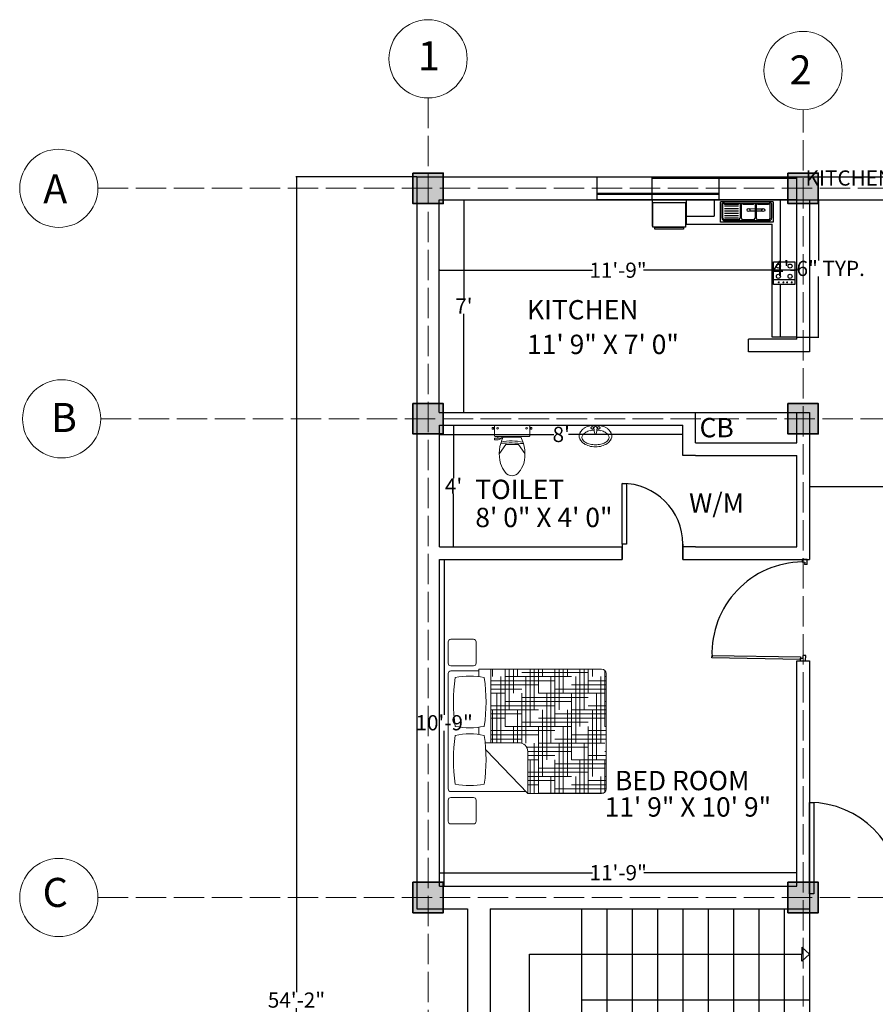
# Model space of a CAD drawing. Units: inches. Extents: x -113 to 5399, y -1393 to 3302.
# Tile 36 of 40: x 3074 to 3412, y 2903 to 3292. Entities that reach past the tile are written whole.
import ezdxf

# ---------------------------------------------------------------- set-up
doc = ezdxf.new("R2010")
doc.units = ezdxf.units.IN
doc.header["$MEASUREMENT"] = 0
doc.linetypes.add('ACAD_ISO02W100', pattern=[15, 12, -3])
for name, color, linetype, lineweight in [('A-ANNO-DIMS', 254, 'Continuous', 18), ('A-AREA-IDEN', 4, 'Continuous', 18), ('A-COLS', 7, 'Continuous', 35), ('A-FLOR-CASE', 8, 'Continuous', 18), ('A-FLOR-FIXT', 8, 'Continuous', 18), ('A-GRID-IDEN', 7, 'Continuous', 18), ('doors', 2, 'Continuous', 25), ('DT TEXT', 4, 'Continuous', 18), ('furniture', 131, 'Continuous', 18), ('GRIDS', 7, 'ACAD_ISO02W100', 13), ('stairs', 210, 'Continuous', 25), ('walls', 1, 'Continuous', 25), ('windows', 3, 'Continuous', 25)]:
    doc.layers.add(name, color=color, linetype=linetype, lineweight=lineweight)
doc.layers.add('TEFRIŞ', color=11, linetype='Continuous')
doc.styles.get("Standard").update_dxf_attribs({"font": 'arial.ttf'})
doc.dimstyles.get("Standard").update_dxf_attribs({"dimtxt": 6, "dimasz": 0.18, "dimexe": 0.18, "dimexo": 0.0625, "dimgap": 0.09, "dimtad": 0, "dimtih": 1, "dimtoh": 1, "dimdec": 1, "dimzin": 0, "dimdsep": 46, "dimlunit": 4, "dimtxsty": 'Standard', "dimblk": 'ARCHTICK', "dimcen": 0.09, "dimadec": 0, "dimazin": 0, "dimtfac": 1, "dimtdec": 1, "dimtofl": 0, "dimtmove": 0, "dimatfit": 3, "dimfxl": 1, "dimtolj": 1, "dimtzin": 0, "dimarcsym": 0})

# ---------------------------------------------------------------- blocks, each defined once
blk = doc.blocks.new('*U2')
for p, q in [((0, 0), (0, -6)), ((24, 0), (24, -6))]:
    blk.add_line(p, q)
blk.add_lwpolyline([(0, 0), (0, 24), (1.75, 24), (1.75, 0)], close=True)
blk.add_arc((0, 0), 24, 0, 90)
blk = doc.blocks.new('*U3')
for p, q in [((0, 0), (0, -6)), ((36, 0), (36, -6))]:
    blk.add_line(p, q)
blk.add_lwpolyline([(0, 0), (0, 36), (1.75, 36), (1.75, 0)], close=True)
blk.add_arc((0, 0), 36, 0, 90)
blk = doc.blocks.new('*X4')
at = {"color": 0}
for p, q in [((4.359, 18.562), (4.359, 18.646)), ((4.453, 17.817), (4.453, 18.562)), ((4.5, 18), (4.5, 18.646)), ((4.5, 18.562), (5.25, 18.562)), ((4.547, 18.188), (4.547, 18.646)), ((4.594, 18.375), (4.594, 18.646)), ((4.641, 18.562), (4.641, 18.646)), ((4.687, 18.609), (5.437, 18.609)), ((4.734, 17.812), (4.734, 18.562)), ((4.781, 18), (4.781, 18.646)), ((4.828, 18.188), (4.828, 18.646)), ((4.875, 18.375), (4.875, 18.646)), ((4.922, 18.562), (4.922, 18.646)), ((5.016, 17.812), (5.016, 18.562)), ((5.062, 18), (5.062, 18.646)), ((5.109, 18.188), (5.109, 18.646)), ((5.156, 18.375), (5.156, 18.646)), ((5.203, 18.562), (5.203, 18.646)), ((5.297, 17.812), (5.297, 18.562)), ((5.344, 18), (5.344, 18.646)), ((5.391, 18.188), (5.391, 18.646)), ((5.437, 18.375), (5.437, 18.646)), ((5.484, 18.562), (5.484, 18.646)), ((5.578, 17.812), (5.578, 18.562)), ((5.625, 18), (5.625, 18.629)), ((5.625, 18.562), (5.637, 18.562)), ((4.34, 18.516), (5.062, 18.516)), ((4.34, 18.469), (4.875, 18.469)), ((5.25, 18.469), (5.637, 18.469)), ((5.437, 18.516), (5.637, 18.516)), ((4.34, 18.422), (4.687, 18.422)), ((4.34, 18.375), (4.5, 18.375)), ((4.406, 17.817), (4.406, 18.375)), ((4.687, 18.328), (5.437, 18.328)), ((4.687, 17.811), (4.687, 18.375)), ((4.875, 18.375), (5.625, 18.375)), ((4.969, 17.625), (4.969, 18.375)), ((5.062, 18.422), (5.637, 18.422)), ((5.25, 17.625), (5.25, 18.375)), ((5.531, 17.625), (5.531, 18.375)), ((4.34, 18.234), (5.062, 18.234)), ((4.5, 18.281), (5.25, 18.281)), ((5.437, 18.234), (5.637, 18.234)), ((5.625, 18.281), (5.637, 18.281)), ((4.34, 18.188), (4.875, 18.188)), ((4.34, 18.141), (4.687, 18.141)), ((4.34, 18.094), (4.5, 18.094)), ((4.359, 17.817), (4.359, 18.188)), ((4.641, 17.817), (4.641, 18.188)), ((4.875, 18.094), (5.625, 18.094)), ((4.922, 17.438), (4.922, 18.188)), ((5.062, 18.141), (5.637, 18.141)), ((5.203, 17.438), (5.203, 18.188)), ((5.25, 18.188), (5.637, 18.188)), ((5.484, 17.438), (5.484, 18.188)), ((4.5, 18), (5.25, 18)), ((4.594, 17.817), (4.594, 18)), ((4.687, 18.047), (5.437, 18.047)), ((4.875, 17.25), (4.875, 18)), ((5.156, 17.25), (5.156, 18)), ((5.437, 17.25), (5.437, 18)), ((5.625, 18), (5.637, 18)), ((4.34, 17.953), (5.062, 17.953)), ((4.34, 17.906), (4.875, 17.906)), ((5.25, 17.906), (5.637, 17.906)), ((5.437, 17.953), (5.637, 17.953)), ((4.34, 17.859), (4.687, 17.859)), ((4.742, 17.766), (5.437, 17.766)), ((4.828, 17.246), (4.828, 17.812)), ((4.875, 17.812), (5.625, 17.812)), ((5.062, 17.859), (5.637, 17.859)), ((5.109, 17.246), (5.109, 17.812)), ((5.391, 17.246), (5.391, 17.812)), ((4.755, 17.719), (5.25, 17.719)), ((4.755, 17.672), (5.062, 17.672)), ((5.437, 17.672), (5.637, 17.672)), ((5.625, 17.719), (5.637, 17.719)), ((4.755, 17.625), (4.875, 17.625)), ((4.781, 17.246), (4.781, 17.625)), ((5.062, 17.246), (5.062, 17.625)), ((5.062, 17.578), (5.637, 17.578)), ((5.25, 17.625), (5.637, 17.625)), ((5.344, 17.246), (5.344, 17.625)), ((5.625, 17.263), (5.625, 17.625)), ((4.755, 17.484), (5.437, 17.484)), ((4.755, 17.438), (5.25, 17.438)), ((4.875, 17.531), (5.625, 17.531)), ((5.016, 17.246), (5.016, 17.438)), ((5.297, 17.246), (5.297, 17.438)), ((5.578, 17.246), (5.578, 17.438)), ((5.625, 17.438), (5.637, 17.438)), ((4.755, 17.391), (5.062, 17.391)), ((4.755, 17.344), (4.875, 17.344)), ((5.25, 17.344), (5.637, 17.344)), ((5.437, 17.391), (5.637, 17.391)), ((4.875, 17.25), (5.608, 17.25)), ((4.969, 17.246), (4.969, 17.25)), ((5.062, 17.297), (5.637, 17.297)), ((5.25, 17.246), (5.25, 17.25)), ((5.531, 17.246), (5.531, 17.25))]:
    blk.add_line(p, q, dxfattribs=at)
blk = doc.blocks.new('MAT-P01')
for p, q in [((-0.021, 0.816), (-0.021, 0.56)), ((0.009, 0.846), (0.247, 0.846)), ((0.277, 0.816), (0.277, 0.56)), ((0.344, 0.816), (0.344, -0.032)), ((0.374, 0.846), (1.674, 0.846)), ((1.704, 0.816), (1.704, 0.5)), ((1.762, 0.816), (1.762, 0.56)), ((1.792, 0.846), (2.031, 0.846)), ((2.061, 0.816), (2.061, 0.56)), ((0.009, 0.53), (0.247, 0.53)), ((0.988, 0.5), (1.069, 0.5)), ((1.639, 0.5), (1.724, 0.5)), ((1.724, 0.5), (1.724, -0.884)), ((1.792, 0.53), (2.031, 0.53)), ((0.815, 0.423), (0.324, -0.051)), ((0.895, 0.429), (0.895, 0.049)), ((0.895, 0.364), (1.724, 0.364)), ((0.895, 0.364), (0.895, 0.049)), ((0.895, 0.364), (1.724, 0.364)), ((1.724, 0.364), (1.724, -0.884)), ((0.324, -0.051), (0.795, -0.051)), ((0.324, -0.051), (0.324, -0.884)), ((0.374, -0.934), (1.674, -0.934))]:
    blk.add_line(p, q)
for centre, radius, start, end in [((0.009, 0.816), 0.03, 90, 180), ((0.247, 0.816), 0.03, 0, 90), ((0.374, 0.816), 0.03, 90, 180), ((0.703, -1.144), 1.931, 81.8162, 98.1838), ((1.354, -1.144), 1.931, 81.8162, 98.1838), ((1.674, 0.816), 0.03, 0, 90), ((1.792, 0.816), 0.03, 90, 180), ((2.031, 0.816), 0.03, 0, 90), ((1.225, 0.603), 0.814, 168.373, 191.627), ((0.181, 0.603), 0.814, 348.373, 11.627), ((1.877, 0.603), 0.814, 168.373, 191.627), ((0.832, 0.603), 0.814, 348.373, 11.627), ((0.009, 0.56), 0.03, 180, 270), ((0.247, 0.56), 0.03, 270, 0), ((1.792, 0.56), 0.03, 180, 270), ((2.031, 0.56), 0.03, 270, 0), ((0.703, 2.35), 1.931, 261.8162, 278.1838), ((1.354, 2.35), 1.931, 261.8162, 278.1838), ((0.795, 0.049), 0.1, 270, 0), ((0.374, -0.884), 0.05, 180, 270), ((1.674, -0.884), 0.05, 270, 0)]:
    blk.add_arc(centre, radius, start, end)
at = {"rotation": 270}
blk.add_blockref('*X4', (-16.922, 4.704), dxfattribs=at)
blk = doc.blocks.new('toilet-3')
at = {"color": 0, "linetype": 'ByBlock'}
for p, q in [((-0.281, -0.05), (-0.281, -0.069)), ((-0.281, -0.05), (-0.261, -0.05)), ((-0.281, -0.069), (-0.261, -0.069)), ((-0.261, -0.047), (-0.261, -0.072)), ((-0.261, -0.047), (-0.251, -0.047)), ((-0.261, -0.072), (-0.251, -0.072)), ((-0.251, -0.047), (-0.251, -0.072)), ((-0.25, -0.03), (-0.25, -0.165)), ((0.24, -0.02), (-0.24, -0.02)), ((0.25, -0.03), (0.25, -0.165)), ((0.261, -0.047), (0.251, -0.047)), ((0.251, -0.047), (0.251, -0.072)), ((0.261, -0.072), (0.251, -0.072)), ((0.261, -0.047), (0.261, -0.072)), ((0.281, -0.05), (0.261, -0.05)), ((0.281, -0.069), (0.261, -0.069)), ((0.281, -0.05), (0.281, -0.069)), ((-0.144, -0.2), (-0.25, -0.2)), ((-0.25, -0.2), (-0.25, -0.222)), ((-0.198, -0.222), (-0.25, -0.222)), ((0.24, -0.175), (-0.24, -0.175)), ((-0.202, -0.2), (-0.202, -0.175)), ((-0.198, -0.222), (-0.16, -0.207)), ((-0.16, -0.207), (-0.16, -0.2)), ((-0.144, -0.2), (-0.144, -0.175)), ((0.125, -0.182), (-0.125, -0.182)), ((-0.089, -0.287), (-0.18, -0.415)), ((0.089, -0.287), (-0.089, -0.287)), ((0.089, -0.287), (0.18, -0.415))]:
    blk.add_line(p, q, dxfattribs=at)
for centre in [(-0.205, -0.059), (0.205, -0.059)]:
    blk.add_circle(centre, 0.0125, dxfattribs=at)
for centre, radius, start, end in [((-0.24, -0.03), 0.01, 90, 180), ((0.24, -0.03), 0.01, 0, 90), ((-0.24, -0.165), 0.01, 180, 270), ((0.376, -0.424), 0.557, 154.2321, 193.6755), ((-0.013, -1.787), 1.521, 83.4552, 95.5271), ((-0.005, -0.896), 0.659, 75.9276, 103.0204), ((-0.376, -0.424), 0.557, 346.3245, 25.7679), ((0.24, -0.165), 0.01, 270, 0), ((0.262, -0.406), 0.452, 199.2942, 217.2549), ((-0.265, -0.4), 0.457, 322.2382, 340.1051), ((-0.001, -0.609), 0.12, 216.3794, 323.6206)]:
    blk.add_arc(centre, radius, start, end, dxfattribs=at)
blk = doc.blocks.new('wash-6')
at = {"color": 0, "linetype": 'ByBlock'}
for p, q in [((-0.036, -0.063), (-0.021, -0.18)), ((0.036, -0.063), (0.021, -0.18))]:
    blk.add_line(p, q, dxfattribs=at)
for centre, radius in [((-0.075, -0.062), 0.0325), ((-0.075, -0.062), 0.0263), ((0.075, -0.062), 0.0325), ((0.075, -0.062), 0.0263)]:
    blk.add_circle(centre, radius, dxfattribs=at)
for centre, radius, start, end in [((0, -0.56), 0.56, 90, 105.4371), ((-0.204, -0.25), 0.17, 148.1465, 180), ((-0.107, -0.311), 0.285, 123.6901, 148.1465), ((-0.217, -0.282), 0.0954, 142.5096, 180), ((-0.114, -0.361), 0.225, 118.369, 142.5096), ((-0.042, -0.407), 0.401, 105.4371, 123.6901), ((-0.045, -0.488), 0.37, 102.6081, 118.369), ((0, -0.69), 0.576, 92.9466, 102.6081), ((0, -0.063), 0.0361, 0, 180), ((0, -0.18), 0.0215, 180, 0), ((0, -0.56), 0.56, 74.5629, 90), ((0, -0.69), 0.576, 77.3919, 87.0534), ((0.045, -0.488), 0.37, 61.631, 77.3919), ((0.042, -0.407), 0.401, 56.3099, 74.5629), ((0.114, -0.361), 0.225, 37.4904, 61.631), ((0.107, -0.311), 0.285, 31.8535, 56.3099), ((0.217, -0.282), 0.0954, 0, 37.4904), ((0.204, -0.25), 0.17, 0, 31.8535), ((-0.204, -0.25), 0.17, 180, 211.8535), ((-0.107, -0.189), 0.285, 211.8535, 236.3099), ((-0.217, -0.282), 0.0954, 180, 217.4904), ((-0.114, -0.203), 0.225, 217.4904, 241.631), ((-0.042, -0.092), 0.401, 236.3099, 254.5629), ((-0.045, -0.076), 0.37, 241.631, 257.3919), ((0, 0.125), 0.576, 257.3919, 270), ((0, 0.125), 0.576, 270, 282.6081), ((0.045, -0.076), 0.37, 282.6081, 298.369), ((0.042, -0.092), 0.401, 285.4371, 303.6901), ((0.114, -0.203), 0.225, 298.369, 322.5096), ((0.107, -0.189), 0.285, 303.6901, 328.1465), ((0.217, -0.282), 0.0954, 322.5096, 0), ((0.204, -0.25), 0.17, 328.1465, 0), ((0, 0.06), 0.56, 254.5629, 270), ((0, 0.06), 0.56, 270, 285.4371)]:
    blk.add_arc(centre, radius, start, end, dxfattribs=at)
blk = doc.blocks.new('_ArchTick')
at = {"color": 0, "linetype": 'ByBlock', "const_width": 0.15}
blk.add_lwpolyline([(-0.5, -0.5), (0.5, 0.5)], dxfattribs=at)
blk = doc.blocks.new('*D130')
at = {"layer": 'A-ANNO-DIMS', "color": 0, "lineweight": -2, "transparency": 16777216}
for p, q in [((3230.48, 3230.06), (3182.83, 3230.06)), ((3183.01, 3230.06), (3183.01, 2908.21)), ((3183.01, 2580.06), (3183.01, 2901.91)), ((3230.48, 2580.06), (3182.83, 2580.06))]:
    blk.add_line(p, q, dxfattribs=at)
at = {"layer": 'Defpoints', "color": 0, "transparency": 16777216}
for p in [(3230.55, 3230.06), (3183.01, 2580.06), (3230.55, 2580.06)]:
    blk.add_point(p, dxfattribs=at)
at = {"layer": 'A-ANNO-DIMS', "color": 0, "lineweight": -2, "transparency": 16777216, "xscale": 0.18, "yscale": 0.18, "zscale": 0.18}
for p, rotation in [((3183.01, 3230.06), 90), ((3183.01, 2580.06), 270)]:
    blk.add_blockref('_ArchTick', p, dxfattribs=dict(at, rotation=rotation))
at = {"layer": 'A-ANNO-DIMS', "color": 0, "transparency": 16777216, "insert": (3183.01, 2905.06), "char_height": 6, "attachment_point": 5}
blk.add_mtext('\\A1;54\'-2"', dxfattribs=at)
blk = doc.blocks.new('*D131')
at = {"layer": 'A-ANNO-DIMS', "color": 0, "lineweight": -2, "transparency": 16777216}
for p, q in [((3239.39, 3193.5), (3239.39, 3193.04)), ((3239.39, 3193.22), (3299.86, 3193.22)), ((3380.55, 3193.22), (3320.08, 3193.22)), ((3380.55, 3193.5), (3380.55, 3193.04))]:
    blk.add_line(p, q, dxfattribs=at)
at = {"layer": 'Defpoints', "color": 0, "transparency": 16777216}
for p in [(3239.39, 3193.56), (3239.39, 3193.22), (3380.55, 3193.56)]:
    blk.add_point(p, dxfattribs=at)
at = {"layer": 'A-ANNO-DIMS', "color": 0, "lineweight": -2, "transparency": 16777216, "xscale": 0.18, "yscale": 0.18, "zscale": 0.18, "rotation": 180}
blk.add_blockref('_ArchTick', (3239.39, 3193.22), dxfattribs=at)
at = {"layer": 'A-ANNO-DIMS', "color": 0, "lineweight": -2, "transparency": 16777216, "xscale": 0.18, "yscale": 0.18, "zscale": 0.18}
blk.add_blockref('_ArchTick', (3380.55, 3193.22), dxfattribs=at)
at = {"layer": 'A-ANNO-DIMS', "color": 0, "transparency": 16777216, "insert": (3309.97, 3193.22), "char_height": 6, "attachment_point": 5}
blk.add_mtext('\\A1;11\'-9"', dxfattribs=at)
blk = doc.blocks.new('*D124')
at = {"layer": 'A-ANNO-DIMS', "color": 0, "lineweight": -2, "transparency": 16777216}
for p, q in [((3249.09, 3221.06), (3249.09, 3182.15)), ((3249.13, 3221.06), (3249.27, 3221.06)), ((3249.09, 3137.06), (3249.09, 3175.97)), ((3249.13, 3137.06), (3249.27, 3137.06))]:
    blk.add_line(p, q, dxfattribs=at)
at = {"layer": 'Defpoints', "color": 0, "transparency": 16777216}
for p in [(3249.07, 3221.06), (3249.07, 3137.06), (3249.09, 3137.06)]:
    blk.add_point(p, dxfattribs=at)
at = {"layer": 'A-ANNO-DIMS', "color": 0, "lineweight": -2, "transparency": 16777216, "xscale": 0.18, "yscale": 0.18, "zscale": 0.18}
for p, rotation in [((3249.09, 3221.06), 90), ((3249.09, 3137.06), 270)]:
    blk.add_blockref('_ArchTick', p, dxfattribs=dict(at, rotation=rotation))
at = {"layer": 'A-ANNO-DIMS', "color": 0, "transparency": 16777216, "insert": (3249.09, 3179.06), "char_height": 6, "attachment_point": 5}
blk.add_mtext("\\A1;7'", dxfattribs=at)
blk = doc.blocks.new('*D126')
at = {"layer": 'A-ANNO-DIMS', "color": 0, "lineweight": -2, "transparency": 16777216}
for p, q in [((3385.55, 3108), (3385.55, 3107.65)), ((3385.55, 3107.83), (3446.65, 3107.83)), ((3517.55, 3107.83), (3456.45, 3107.83)), ((3517.55, 3108), (3517.55, 3107.65))]:
    blk.add_line(p, q, dxfattribs=at)
at = {"layer": 'Defpoints', "color": 0, "transparency": 16777216}
for p in [(3385.55, 3108.06), (3517.55, 3108.06), (3517.55, 3107.83)]:
    blk.add_point(p, dxfattribs=at)
at = {"layer": 'A-ANNO-DIMS', "color": 0, "lineweight": -2, "transparency": 16777216, "xscale": 0.18, "yscale": 0.18, "zscale": 0.18, "rotation": 180}
blk.add_blockref('_ArchTick', (3385.55, 3107.83), dxfattribs=at)
at = {"layer": 'A-ANNO-DIMS', "color": 0, "lineweight": -2, "transparency": 16777216, "xscale": 0.18, "yscale": 0.18, "zscale": 0.18}
blk.add_blockref('_ArchTick', (3517.55, 3107.83), dxfattribs=at)
at = {"layer": 'A-ANNO-DIMS', "color": 0, "transparency": 16777216, "insert": (3451.55, 3107.83), "char_height": 6, "attachment_point": 5}
blk.add_mtext("\\A1;11'", dxfattribs=at)
blk = doc.blocks.new('*D132')
at = {"layer": 'A-ANNO-DIMS', "color": 0, "lineweight": -2, "transparency": 16777216}
for p, q in [((3244.24, 3132.06), (3245.22, 3132.06)), ((3245.04, 3132.06), (3245.04, 3111.15)), ((3245.04, 3084.06), (3245.04, 3104.97)), ((3244.24, 3084.06), (3245.22, 3084.06))]:
    blk.add_line(p, q, dxfattribs=at)
at = {"layer": 'Defpoints', "color": 0, "transparency": 16777216}
for p in [(3244.17, 3132.06), (3244.17, 3084.06), (3245.04, 3084.06)]:
    blk.add_point(p, dxfattribs=at)
at = {"layer": 'A-ANNO-DIMS', "color": 0, "lineweight": -2, "transparency": 16777216, "xscale": 0.18, "yscale": 0.18, "zscale": 0.18}
for p, rotation in [((3245.04, 3132.06), 90), ((3245.04, 3084.06), 270)]:
    blk.add_blockref('_ArchTick', p, dxfattribs=dict(at, rotation=rotation))
at = {"layer": 'A-ANNO-DIMS', "color": 0, "transparency": 16777216, "insert": (3245.04, 3108.06), "char_height": 6, "attachment_point": 5}
blk.add_mtext("\\A1;4'", dxfattribs=at)
blk = doc.blocks.new('*D133')
at = {"layer": 'A-ANNO-DIMS', "color": 0, "lineweight": -2, "transparency": 16777216}
for p, q in [((3239.55, 3128.45), (3239.55, 3128.57)), ((3239.55, 3128.39), (3284.69, 3128.39)), ((3335.55, 3128.39), (3290.4, 3128.39)), ((3335.55, 3128.45), (3335.55, 3128.57))]:
    blk.add_line(p, q, dxfattribs=at)
at = {"layer": 'Defpoints', "color": 0, "transparency": 16777216}
for p in [(3239.55, 3128.39), (3335.55, 3128.39), (3335.55, 3128.39)]:
    blk.add_point(p, dxfattribs=at)
at = {"layer": 'A-ANNO-DIMS', "color": 0, "lineweight": -2, "transparency": 16777216, "xscale": 0.18, "yscale": 0.18, "zscale": 0.18, "rotation": 180}
blk.add_blockref('_ArchTick', (3239.55, 3128.39), dxfattribs=at)
at = {"layer": 'A-ANNO-DIMS', "color": 0, "lineweight": -2, "transparency": 16777216, "xscale": 0.18, "yscale": 0.18, "zscale": 0.18}
blk.add_blockref('_ArchTick', (3335.55, 3128.39), dxfattribs=at)
at = {"layer": 'A-ANNO-DIMS', "color": 0, "transparency": 16777216, "insert": (3287.55, 3128.39), "char_height": 6, "attachment_point": 5}
blk.add_mtext("\\A1;8'", dxfattribs=at)
blk = doc.blocks.new('*D134')
at = {"layer": 'A-ANNO-DIMS', "color": 0, "lineweight": -2, "transparency": 16777216}
for p, q in [((3241.33, 3079.06), (3241.33, 3017.71)), ((3241.39, 3079.06), (3241.51, 3079.06)), ((3241.33, 2950.06), (3241.33, 3011.41)), ((3241.39, 2950.06), (3241.51, 2950.06))]:
    blk.add_line(p, q, dxfattribs=at)
at = {"layer": 'Defpoints', "color": 0, "transparency": 16777216}
for p in [(3241.33, 3079.06), (3241.33, 2950.06), (3241.33, 2950.06)]:
    blk.add_point(p, dxfattribs=at)
at = {"layer": 'A-ANNO-DIMS', "color": 0, "lineweight": -2, "transparency": 16777216, "xscale": 0.18, "yscale": 0.18, "zscale": 0.18}
for p, rotation in [((3241.33, 3079.06), 90), ((3241.33, 2950.06), 270)]:
    blk.add_blockref('_ArchTick', p, dxfattribs=dict(at, rotation=rotation))
at = {"layer": 'A-ANNO-DIMS', "color": 0, "transparency": 16777216, "insert": (3241.33, 3014.56), "char_height": 6, "attachment_point": 5}
blk.add_mtext('\\A1;10\'-9"', dxfattribs=at)
blk = doc.blocks.new('*D135')
at = {"layer": 'A-ANNO-DIMS', "color": 0, "lineweight": -2, "transparency": 16777216}
for p, q in [((3239.55, 2954.85), (3239.55, 2955.53)), ((3239.55, 2955.35), (3299.93, 2955.35)), ((3380.55, 2955.35), (3320.16, 2955.35)), ((3380.55, 2954.85), (3380.55, 2955.53))]:
    blk.add_line(p, q, dxfattribs=at)
at = {"layer": 'Defpoints', "color": 0, "transparency": 16777216}
for p in [(3239.55, 2954.79), (3380.55, 2955.35), (3380.55, 2954.79)]:
    blk.add_point(p, dxfattribs=at)
at = {"layer": 'A-ANNO-DIMS', "color": 0, "lineweight": -2, "transparency": 16777216, "xscale": 0.18, "yscale": 0.18, "zscale": 0.18, "rotation": 180}
blk.add_blockref('_ArchTick', (3239.55, 2955.35), dxfattribs=at)
at = {"layer": 'A-ANNO-DIMS', "color": 0, "lineweight": -2, "transparency": 16777216, "xscale": 0.18, "yscale": 0.18, "zscale": 0.18}
blk.add_blockref('_ArchTick', (3380.55, 2955.35), dxfattribs=at)
at = {"layer": 'A-ANNO-DIMS', "color": 0, "transparency": 16777216, "insert": (3310.05, 2955.35), "char_height": 6, "attachment_point": 5}
blk.add_mtext('\\A1;11\'-9"', dxfattribs=at)
blk = doc.blocks.new('A$C008029BD')
at = {"layer": 'TEFRIŞ', "ltscale": 0.05}
for p, q in [((0, 0), (0, -3.55)), ((3.37, 0), (0, 0)), ((3.37, 0), (3.37, -0.6)), ((1.522, -0.4), (0, -0.4)), ((3.37, -0.4), (2.083, -0.4)), ((0.05, -0.581), (0.05, -1.869)), ((0.05, -0.581), (0.55, -0.581)), ((0.086, -1.773), (0.086, -0.677)), ((0.096, -0.617), (0.454, -0.617)), ((0.099, -0.659), (0.457, -0.659)), ((0.113, -0.954), (0.113, -0.695)), ((0.493, -0.695), (0.493, -0.954)), ((0.514, -0.677), (0.514, -1.773)), ((0.55, -0.581), (0.55, -1.869)), ((0.6, -2.71), (0.6, -0.6)), ((3.37, -0.6), (0.6, -0.6)), ((0.23, -0.846), (0.229, -0.967)), ((0.28, -0.846), (0.277, -1.158)), ((0.096, -1.024), (0.454, -1.024)), ((0.457, -0.99), (0.099, -0.99)), ((0.11, -1.319), (0.11, -1.06)), ((0.228, -1.02), (0.227, -1.159)), ((0.49, -1.06), (0.49, -1.319)), ((0.454, -1.355), (0.096, -1.355)), ((0.096, -1.391), (0.454, -1.391)), ((0.11, -1.773), (0.11, -1.427)), ((0.154, -1.773), (0.154, -1.427)), ((0.214, -1.773), (0.214, -1.427)), ((0.274, -1.773), (0.274, -1.427)), ((0.334, -1.773), (0.334, -1.427)), ((0.39, -1.773), (0.39, -1.427)), ((0.444, -1.773), (0.444, -1.427)), ((0.49, -1.427), (0.49, -1.773)), ((0.55, -1.869), (0.05, -1.869)), ((0.454, -1.809), (0.096, -1.809)), ((0.454, -1.833), (0.096, -1.833)), ((0, -2.025), (0.4, -2.025)), ((0.4, -2.71), (0.4, -2.025)), ((0, -2.71), (0.6, -2.71)), ((0, -3.55), (0.65, -3.55))]:
    blk.add_line(p, q, dxfattribs=at)
at = {"layer": 'TEFRIŞ'}
blk.add_line((1.969, -0.05), (1.969, -0.572), dxfattribs=at)
at = {"layer": 'TEFRIŞ', "ltscale": 0.05}
for points in [[(1.522, -0.05), (2.083, -0.05), (2.083, -0.572), (1.522, -0.572)], [(0.67, -2.73), (0.67, -3.53), (0.07, -3.53), (0.07, -2.73)], [(0.72, -2.78), (0.72, -3.48), (0.67, -3.48), (0.67, -2.78)]]:
    blk.add_lwpolyline(points, close=True, dxfattribs=at)
at = {"layer": 'TEFRIŞ', "const_width": 0.025}
for points in [[(2.014, -0.123, 1), (2.039, -0.123, 1)], [(2.014, -0.236, 1), (2.039, -0.236, 1)], [(2.014, -0.327, 1), (2.039, -0.327, 1)], [(2.014, -0.44, 1), (2.039, -0.44, 1)]]:
    blk.add_lwpolyline(points, format="xyb", close=True, dxfattribs=at)
at = {"layer": 'TEFRIŞ', "ltscale": 0.05}
for centre, radius in [((1.628, -0.164), 0.0505), ((1.628, -0.45), 0.0505), ((0.255, -0.82), 0.036), ((0.252, -1.184), 0.036)]:
    blk.add_circle(centre, radius, dxfattribs=at)
at = {"layer": 'TEFRIŞ'}
for centre in [(1.88, -0.164), (1.88, -0.45)]:
    blk.add_circle(centre, 0.0505, dxfattribs=at)
at = {"layer": 'TEFRIŞ', "ltscale": 0.05}
for centre, radius, start, end in [((0.108, -0.649), 0.0351, 110.4976, 230.5777), ((0.118, -0.673), 0.023, 143.9853, 258.5157), ((0.454, -0.677), 0.06, 0, 90), ((0.457, -0.695), 0.036, 0, 90), ((0.118, -0.976), 0.023, 101.4843, 216.0147), ((0.457, -0.954), 0.036, 270, 0), ((0.115, -1.038), 0.023, 143.9853, 258.5157), ((0.454, -1.06), 0.036, 0, 90), ((0.115, -1.341), 0.023, 101.4843, 216.0147), ((0.115, -1.405), 0.023, 143.9853, 258.5157), ((0.454, -1.319), 0.036, 270, 0), ((0.454, -1.427), 0.036, 0, 90), ((0.108, -1.801), 0.0351, 129.4223, 249.5024), ((0.115, -1.796), 0.023, 101.4843, 216.0147), ((0.454, -1.773), 0.06, 270, 0), ((0.454, -1.773), 0.036, 270, 0)]:
    blk.add_arc(centre, radius, start, end, dxfattribs=at)
blk = doc.blocks.new('WIN-PLAN-48IN')
h = blk.add_hatch(color=256)
h.dxf.hatch_style = 1
h.paths.add_polyline_path([(48, 2.5), (0, 2.5), (0, 2), (48, 2)])
for p, q in [((0, 9), (48, 9)), ((0, 0), (0, 9)), ((48, 9), (48, 0)), ((48, 2.5), (0, 2.5)), ((48, 2), (0, 2)), ((48, 0), (0, 0))]:
    blk.add_line(p, q)
blk = doc.blocks.new('COLUMN-12IN-SQUARE')
h = blk.add_hatch(color=256)
h.dxf.hatch_style = 1
h.paths.add_polyline_path([(6, 6), (-6, 6), (-6, -6), (6, -6)])
blk.add_lwpolyline([(-6, 6), (6, 6), (6, -6), (-6, -6)], close=True)
blk = doc.blocks.new('STAIR-RESIDENTIAL-PLAN')
for p, q in [((20.54, 72), (20.54, 0)), ((30.54, 72), (30.54, 0)), ((40.54, 72), (40.54, 0)), ((50.54, 72), (50.54, 0)), ((60.54, 72), (60.54, 0)), ((70.54, 72), (70.54, 0)), ((80.54, 72), (80.54, 0)), ((90.54, 72), (90.54, 0)), ((100.54, 72), (100.54, 0)), ((110.54, 72), (110.54, 0)), ((110.54, 54.14), (107.61, 56.9)), ((107.61, 56.9), (107.61, 54.14)), ((0, 17.09), (0, 54.14)), ((0, 54.14), (107.61, 54.14)), ((110.54, 54.14), (107.61, 51.38)), ((107.61, 51.38), (107.61, 54.14)), ((110.54, 36), (20.54, 36)), ((110.54, 17.09), (0, 17.09))]:
    blk.add_line(p, q)
blk = doc.blocks.new('DOOR-SINGLE-36IN-PLAN')
for p, q in [((0.5, 2), (0.5, 36.98)), ((0.5, 36.98), (1.5, 36.98)), ((1.5, 36.98), (1.5, 2)), ((0, 2), (0, 0)), ((0, 2), (1.04, 2)), ((1.5, 2), (0.5, 2)), ((1.04, 2), (1.04, 0.98)), ((1.04, 0.98), (2, 0.98)), ((2, 0), (2, 0.98)), ((38.96, 0.98), (38, 0.98)), ((38, 0), (38, 0.98)), ((40, 2), (38.96, 2)), ((38.96, 2), (38.96, 0.98)), ((40, 0), (40, 2)), ((0, 0), (2, 0)), ((0, 0), (2, 0)), ((38, 0), (40, 0))]:
    blk.add_line(p, q)
blk.add_arc((2.94, 0.99), 36.04, 1.6003, 93.0893)
blk = doc.blocks.new('GRID-BUBBLE-A')
blk.add_circle((0, 0), 15.44)
blk.add_text('A', height=11.45).set_placement((-6.15, -5.94))
blk = doc.blocks.new('GRID-BUBBLE-B')
blk.add_circle((0, 0), 15.44)
blk.add_text('B', height=11.45).set_placement((-4.23, -5.2))
blk = doc.blocks.new('GRID-BUBBLE-C')
blk.add_circle((0, 0), 15.44)
blk.add_text('C', height=11.45).set_placement((-6.38, -3.72))
blk = doc.blocks.new('GRID-BUBBLE-1')
blk.add_circle((0, 0), 15.44)
blk.add_text('1', height=11.45).set_placement((-3.99, -4.52))
blk = doc.blocks.new('GRID-BUBBLE-2')
blk.add_circle((0, 0), 15.44)
blk.add_text('2', height=11.45).set_placement((-5.33, -5.46))
blk = doc.blocks.new('*D181')
at = {"layer": 'A-ANNO-DIMS', "color": 0, "lineweight": -2, "transparency": 16777216}
for p, q in [((3323.4, 3221.12), (3323.4, 3229.81)), ((3323.4, 3229.63), (3380.55, 3229.63)), ((3380.55, 3221.12), (3380.55, 3229.81)), ((3380.55, 3229.63), (3380.73, 3229.63))]:
    blk.add_line(p, q, dxfattribs=at)
at = {"layer": 'Defpoints', "color": 0, "transparency": 16777216}
for p in [(3380.55, 3229.63), (3323.4, 3221.06), (3380.55, 3221.06)]:
    blk.add_point(p, dxfattribs=at)
at = {"layer": 'A-ANNO-DIMS', "color": 0, "lineweight": -2, "transparency": 16777216, "xscale": 0.18, "yscale": 0.18, "zscale": 0.18, "rotation": 180}
blk.add_blockref('_ArchTick', (3323.4, 3229.63), dxfattribs=at)
at = {"layer": 'A-ANNO-DIMS', "color": 0, "lineweight": -2, "transparency": 16777216, "xscale": 0.18, "yscale": 0.18, "zscale": 0.18}
blk.add_blockref('_ArchTick', (3380.55, 3229.63), dxfattribs=at)
at = {"layer": 'A-ANNO-DIMS', "color": 0, "transparency": 16777216, "insert": (3440.42, 3229.63), "char_height": 6, "attachment_point": 5}
blk.add_mtext('\\A1;KITCHEN COUNTER 4\'-9" TYP.', dxfattribs=at)
blk = doc.blocks.new('*D182')
at = {"layer": 'A-ANNO-DIMS', "color": 0, "lineweight": -2, "transparency": 16777216}
for p, q in [((3380.61, 3221.06), (3389.3, 3221.06)), ((3389.12, 3221.06), (3389.12, 3197.09)), ((3389.12, 3166.81), (3389.12, 3190.78)), ((3380.61, 3166.81), (3389.3, 3166.81))]:
    blk.add_line(p, q, dxfattribs=at)
at = {"layer": 'Defpoints', "color": 0, "transparency": 16777216}
for p in [(3380.55, 3221.06), (3380.55, 3166.81), (3389.12, 3166.81)]:
    blk.add_point(p, dxfattribs=at)
at = {"layer": 'A-ANNO-DIMS', "color": 0, "lineweight": -2, "transparency": 16777216, "xscale": 0.18, "yscale": 0.18, "zscale": 0.18}
for p, rotation in [((3389.12, 3221.06), 90), ((3389.12, 3166.81), 270)]:
    blk.add_blockref('_ArchTick', p, dxfattribs=dict(at, rotation=rotation))
at = {"layer": 'A-ANNO-DIMS', "color": 0, "transparency": 16777216, "insert": (3389.12, 3193.93), "char_height": 6, "attachment_point": 5}
blk.add_mtext('\\A1;4\'-6" TYP.', dxfattribs=at)

msp = doc.modelspace()

# ---------------------------------------------------------------- linework, layer by layer
at = {"layer": 'GRIDS'}
for p, q in [((3234.97, 3261.26), (3234.97, 2482.84)), ((3383.05, 2497.57), (3383.05, 3256.61)), ((3104.61, 3225.56), (3753.5, 3225.56)), ((3105.74, 3134.56), (3762.86, 3134.56)), ((3104.61, 2945.56), (3762.86, 2945.56))]:
    msp.add_line(p, q, dxfattribs=at)
at = {"layer": 'walls'}
for p, q in [((3230.55, 3230.06), (3230.55, 2941.06)), ((3230.55, 3230.06), (3427.55, 3230.06)), ((3239.39, 3221.06), (3301.8, 3221.06)), ((3239.39, 3137.06), (3239.39, 3221.06)), ((3271.05, 3221.06), (3380.55, 3221.06)), ((3380.55, 3166.06), (3380.55, 3221.06)), ((3385.55, 3221.06), (3385.55, 3161.06)), ((3385.55, 3221.06), (3427.55, 3221.06)), ((3380.55, 3166.06), (3361.55, 3166.06)), ((3361.55, 3161.06), (3361.55, 3166.06)), ((3385.55, 3161.06), (3361.55, 3161.06)), ((3239.39, 3137.06), (3266.05, 3137.06)), ((3266.05, 3137.06), (3271.05, 3137.06)), ((3271.05, 3137.06), (3380.55, 3137.06)), ((3340.55, 3125.06), (3340.55, 3137.06)), ((3380.55, 3125.06), (3380.55, 3137.06)), ((3380.55, 3137.06), (3385.55, 3137.06)), ((3385.55, 3137.06), (3385.55, 3079.06)), ((3239.55, 3084.06), (3239.55, 3132.06)), ((3239.55, 3132.06), (3335.55, 3132.06)), ((3335.55, 3120.06), (3335.55, 3132.06)), ((3340.55, 3125.06), (3380.55, 3125.06)), ((3340.55, 3120.06), (3335.55, 3120.06)), ((3340.55, 3120.06), (3380.55, 3120.06)), ((3380.55, 3084.06), (3380.55, 3120.06)), ((3239.55, 3084.06), (3311.55, 3084.06)), ((3311.55, 3079.06), (3311.55, 3084.06)), ((3335.55, 3079.06), (3335.55, 3085.06)), ((3340.55, 3084.06), (3335.55, 3084.06)), ((3340.55, 3084.06), (3380.55, 3084.06)), ((3239.55, 2950.06), (3239.55, 3079.06)), ((3239.55, 3079.06), (3311.55, 3079.06)), ((3335.55, 3079.06), (3380.55, 3079.06)), ((3380.55, 3079.06), (3385.55, 3079.06)), ((3380.55, 2950.06), (3380.55, 3039.06)), ((3380.55, 3039.06), (3385.55, 3039.06)), ((3385.55, 3039.06), (3385.55, 2950.06)), ((3239.55, 2950.06), (3380.55, 2950.06)), ((3385.55, 2950.06), (3385.55, 2941.06)), ((3230.55, 2941.06), (3250.55, 2941.06)), ((3250.55, 2941.06), (3250.55, 2869.06)), ((3259.55, 2941.06), (3385.55, 2941.06)), ((3259.55, 2941.06), (3259.55, 2869.06))]:
    msp.add_line(p, q, dxfattribs=at)

# ---------------------------------------------------------------- block references
at = {"layer": 'A-COLS'}
for p in [(3234.97, 3225.56), (3383.05, 3225.56), (3234.97, 3134.56), (3383.05, 3134.56), (3234.97, 2945.56), (3383.05, 2945.56)]:
    msp.add_blockref('COLUMN-12IN-SQUARE', p, dxfattribs=at)
at = {"layer": 'A-FLOR-CASE', "xscale": 16.09806929200166, "yscale": 16.09806929200166, "zscale": 16.09806929200166, "rotation": 270}
msp.add_blockref('A$C008029BD', (3380.55, 3221.06), dxfattribs=at)
at = {"layer": 'A-FLOR-FIXT'}
for name, p, xscale, yscale, zscale in [('toilet-3', (3268.15, 3132.46), 27.95492935005888, 27.95492935005888, 27.95492935005888), ('wash-6', (3301.09, 3132.06), 17.16666334294967, 17.16666334294967, 17.16666334294967)]:
    msp.add_blockref(name, p, dxfattribs=dict(at, xscale=xscale, yscale=yscale, zscale=zscale))
at = {"layer": 'A-GRID-IDEN'}
for name, p in [('GRID-BUBBLE-1', (3234.97, 3276.7)), ('GRID-BUBBLE-2', (3383.05, 3272.05)), ('GRID-BUBBLE-A', (3089.17, 3225.56)), ('GRID-BUBBLE-B', (3090.3, 3134.56)), ('GRID-BUBBLE-C', (3089.17, 2945.56))]:
    msp.add_blockref(name, p, dxfattribs=at)
at = {"layer": 'doors'}
for name, p in [('*U2', (3311.55, 3085.06)), ('*U3', (3385.55, 2947.06))]:
    msp.add_blockref(name, p, dxfattribs=at)
at = {"layer": 'doors', "rotation": 89.09244041658943}
msp.add_blockref('DOOR-SINGLE-36IN-PLAN', (3384.05, 3039.04), dxfattribs=at)
at = {"layer": 'furniture', "xscale": 35.02364872074636, "yscale": 35.02364872074636, "zscale": 35.02364872074636, "rotation": 90}
msp.add_blockref('MAT-P01', (3272.54, 2975.32), dxfattribs=at)
at = {"layer": 'stairs'}
msp.add_blockref('STAIR-RESIDENTIAL-PLAN', (3275.01, 2869.06), dxfattribs=at)
at = {"layer": 'windows'}
msp.add_blockref('WIN-PLAN-48IN', (3301.8, 3221.06), dxfattribs=at)

# ---------------------------------------------------------------- texts
at = {"layer": 'A-AREA-IDEN'}
for s, height, p in [('KITCHEN', 7.647, (3274.06, 3173.79)), ('11\' 9" X 7\' 0"', 7.6473, (3274.06, 3160.12)), ('TOILET', 7.647, (3253.63, 3102.87)), ('8\' 0" X 4\' 0"', 7.6473, (3253.63, 3091.78)), ('BED ROOM', 7.647, (3308.79, 2987.91)), ('11\' 9" X 10\' 9"', 7.6473, (3304.68, 2977.49))]:
    msp.add_text(s, height=height, dxfattribs=at).set_placement(p)
at = {"layer": 'DT TEXT'}
for s, p in [('CB', (3342.17, 3127.25)), (' W/M', (3335.7, 3097.5))]:
    msp.add_text(s, height=7.647, dxfattribs=at).set_placement(p)

# ---------------------------------------------------------------- dimensions: what is measured, and where the dimension line sits
at = {"layer": 'A-ANNO-DIMS'}
dim = msp.add_linear_dim(base=(3380.5461, 3229.6314), p1=(3323.398, 3221.0592), p2=(3380.5461, 3221.0592), text='KITCHEN COUNTER <> TYP.', dimstyle='Standard', override={"dimdec": 1, "dimlfac": 1, "dimrnd": 0, "dimzin": 1, "dimdsep": 46, "dimlunit": 4, "dimfrac": 2}, dxfattribs=at)
dim.commit()
dim.dimension.update_dxf_attribs({"geometry": '*D181', "text_midpoint": (3440.415, 3229.6314)})
for base, p1, p2, picture, middle in [((3183.01, 2580.06), (3230.55, 3230.06), (3230.55, 2580.06), '*D130', (3183.01, 2905.06)), ((3245.04, 3084.06), (3244.17, 3132.06), (3244.17, 3084.06), '*D132', (3245.04, 3108.06)), ((3241.33, 2950.06), (3241.33, 3079.06), (3241.33, 2950.06), '*D134', (3241.33, 3014.56))]:
    dim = msp.add_linear_dim(base=base, p1=p1, p2=p2, angle=90, dimstyle='Standard', override={"dimclrd": 0, "dimclre": 0, "dimclrt": 0}, dxfattribs=at)
    dim.commit()
    dim.dimension.update_dxf_attribs({"geometry": picture, "text_midpoint": middle})
dim = msp.add_linear_dim(base=(3249.09, 3137.06), p1=(3249.07, 3221.06), p2=(3249.07, 3137.06), angle=90, dimstyle='Standard', override={"dimclrd": 0, "dimclre": 0, "dimclrt": 0}, dxfattribs=at)
dim.commit()
dim.dimension.update_dxf_attribs({"geometry": '*D124', "text_midpoint": (3249.09, 3179.06), "dimtype": 160})
dim = msp.add_linear_dim(base=(3389.1183, 3166.81), p1=(3380.5461, 3221.0592), p2=(3380.5461, 3166.81), angle=270, text='<> TYP.', dimstyle='Standard', override={"dimdec": 1, "dimlfac": 1, "dimrnd": 0, "dimzin": 1, "dimdsep": 46, "dimlunit": 4, "dimfrac": 2}, dxfattribs=at)
dim.commit()
dim.dimension.update_dxf_attribs({"geometry": '*D182', "text_midpoint": (3389.1183, 3193.9346)})
for base, p1, p2, picture, middle in [((3239.39, 3193.22), (3380.55, 3193.56), (3239.39, 3193.56), '*D131', (3309.97, 3193.22)), ((3335.55, 3128.39), (3239.55, 3128.39), (3335.55, 3128.39), '*D133', (3287.55, 3128.39)), ((3517.55, 3107.83), (3385.55, 3108.06), (3517.55, 3108.06), '*D126', (3451.55, 3107.83)), ((3380.55, 2955.35), (3239.55, 2954.79), (3380.55, 2954.79), '*D135', (3310.05, 2955.35))]:
    dim = msp.add_linear_dim(base=base, p1=p1, p2=p2, dimstyle='Standard', override={"dimclrd": 0, "dimclre": 0, "dimclrt": 0}, dxfattribs=at)
    dim.commit()
    dim.dimension.update_dxf_attribs({"geometry": picture, "text_midpoint": middle})

doc.saveas('drawing.dxf')
